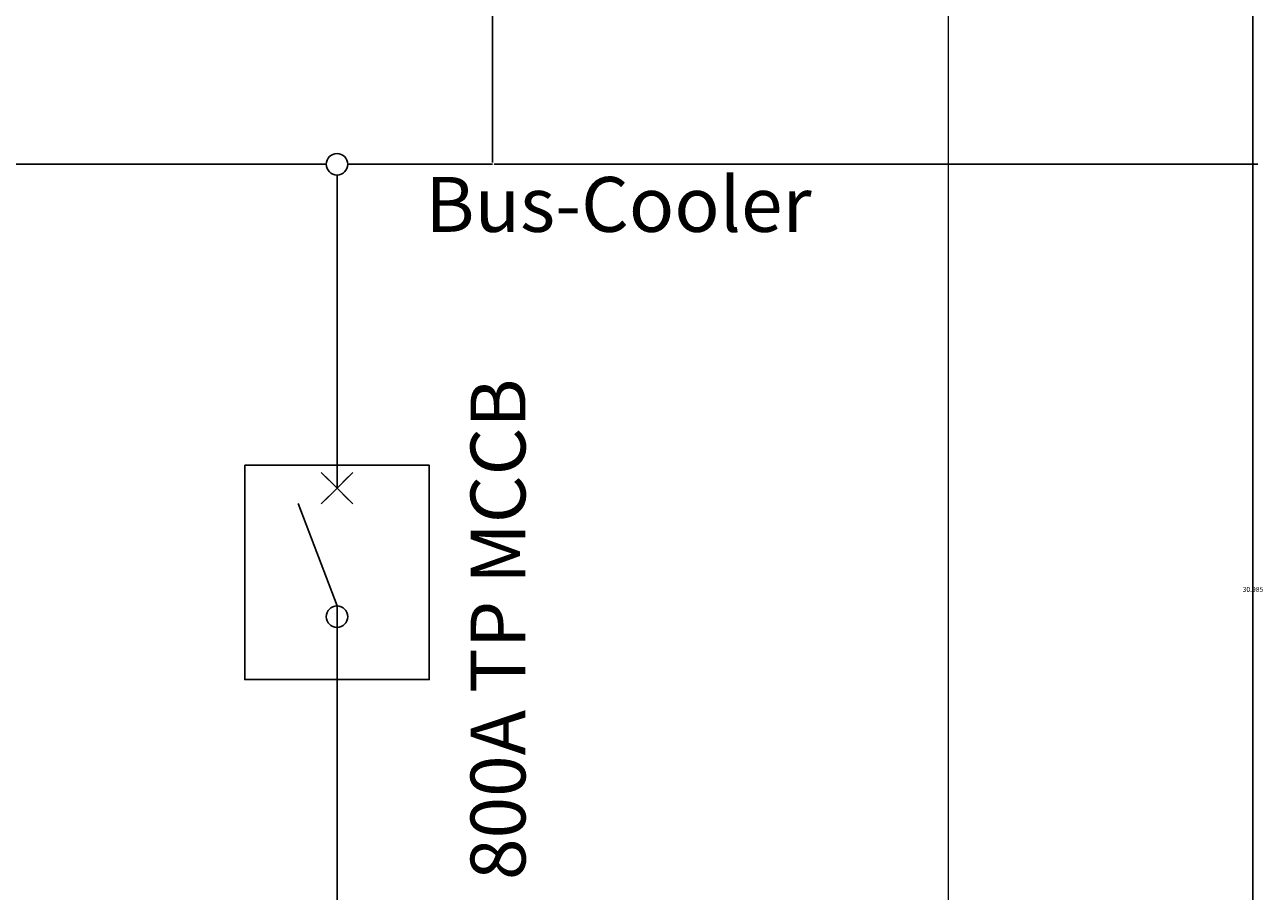
# Model space of a CAD drawing. Units: inches. Extents: x 412 to 584, y 208 to 437.
# Tile 10 of 28: x 539 to 584, y 230 to 262. Entities that reach past the tile are written whole.
import ezdxf

# ---------------------------------------------------------------- set-up
doc = ezdxf.new("R2010")
doc.units = ezdxf.units.IN
doc.header["$MEASUREMENT"] = 0
for name, color, linetype, lineweight in [('A-ANNO-DIMS', 2, 'Continuous', 18), ('E-ANNO-TEXT', 7, 'Continuous', 18), ('E-ENCL', 8, 'Continuous', 18), ('E-POWR-EQPM', 3, 'Continuous', 25)]:
    doc.layers.add(name, color=color, linetype=linetype, lineweight=lineweight)
doc.styles.get("Standard").update_dxf_attribs({"font": 'arial.ttf'})
doc.dimstyles.get("Standard").update_dxf_attribs({"dimtxt": 0.18, "dimasz": 0.18, "dimexe": 0.18, "dimexo": 0.0625, "dimgap": 0.09, "dimtad": 0, "dimtih": 1, "dimtoh": 1, "dimdec": 4, "dimzin": 0, "dimdsep": 46, "dimtxsty": 'Standard', "dimcen": 0.09, "dimadec": 0, "dimazin": 0, "dimtfac": 1, "dimtdec": 4, "dimtofl": 0, "dimtmove": 0, "dimatfit": 3, "dimfxl": 1, "dimtolj": 1, "dimtzin": 0, "dimarcsym": 0})

# ---------------------------------------------------------------- blocks, each defined once
blk = doc.blocks.new('*U3')
blk.add_line((-0.212, 0.212), (0.212, -0.212))
blk = doc.blocks.new('*U4')
at = {"color": 0, "linetype": 'ByBlock', "lineweight": -2, "transparency": 16777216}
for p, rotation in [((224.254, 56.203), 180), ((224.677, 56.203), 89.99999999999999), ((224.254, 55.78), 269.9999999999999)]:
    blk.add_blockref('*U3', p, dxfattribs=dict(at, rotation=rotation))
blk.add_blockref('*U3', (224.677, 55.78), dxfattribs=at)
blk = doc.blocks.new('*U7')
blk.add_line((-0.288, 0.288), (0.288, -0.288))
blk = doc.blocks.new('*U8')
at = {"color": 0, "linetype": 'ByBlock', "lineweight": -2, "transparency": 16777216}
for p, rotation in [((224.177, 56.28), 180), ((224.754, 56.28), 90), ((224.177, 55.703), 269.9999999999999)]:
    blk.add_blockref('*U7', p, dxfattribs=dict(at, rotation=rotation))
blk.add_blockref('*U7', (224.754, 55.703), dxfattribs=at)
blk = doc.blocks.new('MCCB-800A')
for q in [(1.94, 18.628), (3.361, 0)]:
    blk.add_line((3.361, 14.893), q)
blk.add_lwpolyline([(0, 20.016), (6.722, 20.016), (6.722, 12.209), (0, 12.209)], close=True)
blk.add_circle((3.361, 14.5), 0.393)
for name in ['*U8', '*U4']:
    blk.add_blockref(name, (-221.104, -36.809))
blk = doc.blocks.new('*D17')
at = {"layer": 'A-ANNO-DIMS', "color": 0, "lineweight": -2, "transparency": 16777216}
for p, q in [((497.715, 426.185), (583.674, 426.185)), ((583.494, 426.005), (583.494, 323.031)), ((583.494, 219.693), (583.494, 322.667)), ((550.198, 219.513), (583.674, 219.513))]:
    blk.add_line(p, q, dxfattribs=at)
at = {"layer": 'A-ANNO-DIMS', "color": 0, "transparency": 16777216}
for points in [[(583.464, 426.005), (583.524, 426.005), (583.494, 426.185)], [(583.464, 219.693), (583.524, 219.693), (583.494, 219.513)]]:
    blk.add_solid(points, dxfattribs=at)
at = {"layer": 'Defpoints', "color": 0, "transparency": 16777216}
for p in [(497.652, 426.185), (550.135, 219.513), (583.494, 219.513)]:
    blk.add_point(p, dxfattribs=at)
at = {"layer": 'A-ANNO-DIMS', "color": 0, "transparency": 16777216, "insert": (583.494, 322.849), "char_height": 0.18, "attachment_point": 5}
blk.add_mtext('\\A1;206.67', dxfattribs=at)
blk = doc.blocks.new('*D18')
at = {"layer": 'A-ANNO-DIMS', "color": 0, "lineweight": -2, "transparency": 16777216}
for p, q in [((572.456, 309.377), (583.674, 309.377)), ((583.494, 309.197), (583.494, 267.665)), ((583.494, 225.768), (583.494, 267.301)), ((572.456, 225.588), (583.674, 225.588))]:
    blk.add_line(p, q, dxfattribs=at)
at = {"layer": 'A-ANNO-DIMS', "color": 0, "transparency": 16777216}
for points in [[(583.464, 309.197), (583.524, 309.197), (583.494, 309.377)], [(583.464, 225.768), (583.524, 225.768), (583.494, 225.588)]]:
    blk.add_solid(points, dxfattribs=at)
at = {"layer": 'Defpoints', "color": 0, "transparency": 16777216}
for p in [(572.394, 309.377), (572.394, 225.588), (583.494, 225.588)]:
    blk.add_point(p, dxfattribs=at)
at = {"layer": 'A-ANNO-DIMS', "color": 0, "transparency": 16777216, "insert": (583.494, 267.483), "char_height": 0.18, "attachment_point": 5}
blk.add_mtext('\\A1;83.79', dxfattribs=at)
blk = doc.blocks.new('*D19')
at = {"layer": 'A-ANNO-DIMS', "color": 0, "lineweight": -2, "transparency": 16777216}
for p, q in [((555.858, 256.573), (583.674, 256.573)), ((583.494, 256.393), (583.494, 241.263)), ((583.494, 225.768), (583.494, 240.899)), ((572.456, 225.588), (583.674, 225.588))]:
    blk.add_line(p, q, dxfattribs=at)
at = {"layer": 'A-ANNO-DIMS', "color": 0, "transparency": 16777216}
for points in [[(583.464, 256.393), (583.524, 256.393), (583.494, 256.573)], [(583.464, 225.768), (583.524, 225.768), (583.494, 225.588)]]:
    blk.add_solid(points, dxfattribs=at)
at = {"layer": 'Defpoints', "color": 0, "transparency": 16777216}
for p in [(555.796, 256.573), (572.394, 225.588), (583.494, 225.588)]:
    blk.add_point(p, dxfattribs=at)
at = {"layer": 'A-ANNO-DIMS', "color": 0, "transparency": 16777216, "insert": (583.494, 241.081), "char_height": 0.18, "attachment_point": 5}
blk.add_mtext('\\A1;30.985', dxfattribs=at)
blk = doc.blocks.new('*D28')
at = {"layer": 'A-ANNO-DIMS', "color": 0, "lineweight": -2, "transparency": 16777216}
for p, q in [((450.562, 256.635), (450.562, 437.465)), ((450.742, 437.285), (502.724, 437.285)), ((555.616, 437.285), (503.634, 437.285)), ((555.796, 256.635), (555.796, 437.465))]:
    blk.add_line(p, q, dxfattribs=at)
at = {"layer": 'A-ANNO-DIMS', "color": 0, "transparency": 16777216}
for points in [[(450.742, 437.315), (450.742, 437.255), (450.562, 437.285)], [(555.616, 437.315), (555.616, 437.255), (555.796, 437.285)]]:
    blk.add_solid(points, dxfattribs=at)
at = {"layer": 'Defpoints', "color": 0, "transparency": 16777216}
for p in [(555.796, 437.285), (450.562, 256.573), (555.796, 256.573)]:
    blk.add_point(p, dxfattribs=at)
at = {"layer": 'A-ANNO-DIMS', "color": 0, "transparency": 16777216, "insert": (503.179, 437.285), "char_height": 0.18, "attachment_point": 5}
blk.add_mtext('\\A1;105.23', dxfattribs=at)

msp = doc.modelspace()

# ---------------------------------------------------------------- linework, layer by layer
at = {"layer": 'E-ENCL'}
msp.add_lwpolyline([(423.5562, 309.3773), (572.3937, 309.3773), (572.3937, 225.5881), (423.5562, 225.5881)], close=True, dxfattribs=at)
at = {"layer": 'E-POWR-EQPM'}
for p, q in [((499.6808, 256.5729), (549.7416, 256.5729)), ((550.5286, 256.5729), (555.7959, 256.5729)), ((550.1351, 256.1795), (550.1351, 244.7702))]:
    msp.add_line(p, q, dxfattribs=at)
msp.add_circle((550.1351, 256.5729), 0.3935, dxfattribs=at)

# ---------------------------------------------------------------- block references
msp.add_blockref('MCCB-800A', (546.774, 225.588), dxfattribs=at)

# ---------------------------------------------------------------- texts
at = {"layer": 'E-ANNO-TEXT', "insert": (553.5684, 256.1112), "char_height": 2, "attachment_point": 1}
msp.add_mtext_dynamic_manual_height_columns('\\pxqc;{Bus-Cooler}', width=13.633448, gutter_width=1, heights=[2.9648], dxfattribs=at)
at = {"layer": 'E-ANNO-TEXT', "insert": (554.9982, 228.1355), "char_height": 2, "attachment_point": 1, "rotation": 90}
msp.add_mtext_dynamic_manual_height_columns('\\pxqc;800A TP MCCB', width=22.986562, gutter_width=1, heights=[7.3417], dxfattribs=at)

# ---------------------------------------------------------------- dimensions: what is measured, and where the dimension line sits
at = {"layer": 'A-ANNO-DIMS'}
dim = msp.add_linear_dim(base=(555.7959, 437.2847), p1=(450.562, 256.5729), p2=(555.7959, 256.5729), dimstyle='Standard', override={"dimdec": 2, "dimlfac": 1, "dimrnd": 0, "dimzin": 0, "dimdsep": 46, "dimlunit": 2}, dxfattribs=at)
dim.commit()
dim.dimension.update_dxf_attribs({"geometry": '*D28', "text_midpoint": (503.1789, 437.2847)})
for base, p1, p2, override, picture, middle in [((583.4937, 219.5133), (497.6523, 426.1847), (550.1351, 219.5133), {"dimdec": 2, "dimlfac": 1, "dimrnd": 0, "dimzin": 0, "dimdsep": 46, "dimlunit": 2}, '*D17', (583.4937, 322.849)), ((583.4937, 225.5881), (572.3937, 309.3773), (572.3937, 225.5881), {"dimdec": 2, "dimlfac": 1, "dimrnd": 0, "dimzin": 0, "dimdsep": 46, "dimlunit": 2}, '*D18', (583.4937, 267.4827)), ((583.4937, 225.5881), (555.7959, 256.5729), (572.3937, 225.5881), {"dimdec": 3, "dimlfac": 1, "dimrnd": 0, "dimzin": 0, "dimdsep": 46, "dimlunit": 2}, '*D19', (583.4937, 241.0805))]:
    dim = msp.add_linear_dim(base=base, p1=p1, p2=p2, angle=90, dimstyle='Standard', override=override, dxfattribs=at)
    dim.commit()
    dim.dimension.update_dxf_attribs({"geometry": picture, "text_midpoint": middle})

doc.saveas('drawing.dxf')
